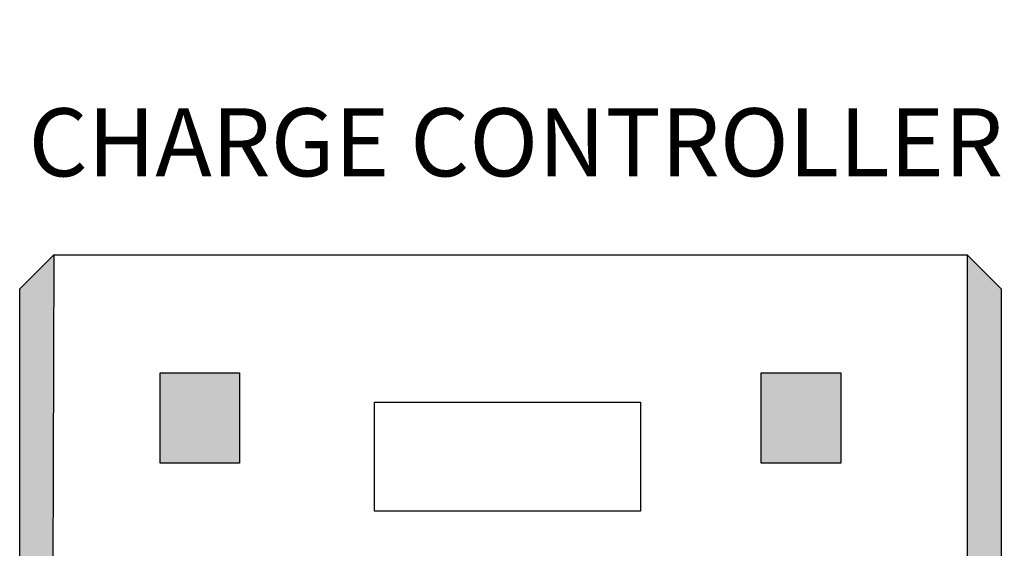
# Model space of a CAD drawing. Units: millimetres. Extents: x -8 to 285, y 5 to 221.
# Tile 7 of 30: x 26 to 84, y 82 to 113. Entities that reach past the tile are written whole.
import ezdxf

# ---------------------------------------------------------------- set-up
doc = ezdxf.new("R2010")
doc.units = ezdxf.units.MM
for name, color, linetype, lineweight in [('A-ANNO-DIMS', 2, 'Continuous', 18), ('E-ANNO-TEXT', 7, 'Continuous', 18), ('E-EQPM-PATT', 252, 'Continuous', 13), ('E-POWR-CTRL', 7, 'Continuous', 30)]:
    doc.layers.add(name, color=color, linetype=linetype, lineweight=lineweight)
doc.styles.get("Standard").update_dxf_attribs({"font": 'arial.ttf'})
doc.dimstyles.get("Standard").update_dxf_attribs({"dimtxt": 0.18, "dimasz": 0.18, "dimexe": 0.18, "dimexo": 0.0625, "dimgap": 0.09, "dimtad": 0, "dimtih": 1, "dimtoh": 1, "dimdec": 4, "dimzin": 0, "dimdsep": 46, "dimtxsty": 'Standard', "dimcen": 0.09, "dimadec": 0, "dimazin": 0, "dimtfac": 1, "dimtdec": 4, "dimtofl": 0, "dimtmove": 0, "dimatfit": 3, "dimfxl": 1, "dimtolj": 1, "dimtzin": 0, "dimarcsym": 0})

# ---------------------------------------------------------------- blocks, each defined once
blk = doc.blocks.new('*D10')
at = {"layer": 'A-ANNO-DIMS', "color": 0, "lineweight": -2, "transparency": 16777216}
for p, q in [((145.103, 206.457), (-7.608, 206.457)), ((-7.428, 206.277), (-7.428, 113.161)), ((-7.428, 19.682), (-7.428, 112.797)), ((30.453, 19.502), (-7.608, 19.502))]:
    blk.add_line(p, q, dxfattribs=at)
at = {"layer": 'A-ANNO-DIMS', "color": 0, "transparency": 16777216}
for points in [[(-7.458, 206.277), (-7.398, 206.277), (-7.428, 206.457)], [(-7.458, 19.682), (-7.398, 19.682), (-7.428, 19.502)]]:
    blk.add_solid(points, dxfattribs=at)
at = {"layer": 'Defpoints', "color": 0, "transparency": 16777216}
for p in [(-7.428, 206.457), (145.165, 206.457), (30.516, 19.502)]:
    blk.add_point(p, dxfattribs=at)
at = {"layer": 'A-ANNO-DIMS', "color": 0, "transparency": 16777216, "insert": (-7.428, 112.979), "char_height": 0.18, "attachment_point": 5}
blk.add_mtext('\\A1;186.95', dxfattribs=at)

msp = doc.modelspace()

# ---------------------------------------------------------------- hatches: boundary and pattern name
at = {"layer": 'E-EQPM-PATT'}
h = msp.add_hatch(color=256, dxfattribs=at)
h.set_gradient(color1=(248, 153, 30), color2=(248, 153, 30), tint=1)
h.paths.add_polyline_path([(28.1554, 99.1437), (26.1554, 97.1437), (26.1554, 65.7282), (28.0483, 63.8353)])
h.paths.add_polyline_path([(81.859, 63.7282), (83.859, 65.7282), (83.859, 97.1437), (81.859, 99.1437)])
h.paths.add_polyline_path([(39.086, 92.2191), (34.4177, 92.2191), (34.4177, 86.904), (39.086, 86.904)])
h.paths.add_polyline_path([(74.424, 86.904), (74.424, 92.2191), (69.7557, 92.2191), (69.7557, 86.904)])
h.paths.add_polyline_path([(74.5326, 81.2093), (69.8643, 81.2093), (69.8643, 75.8943), (74.5326, 75.8943)])
h.paths.add_polyline_path([(34.4177, 75.3519), (39.086, 75.3519), (39.086, 80.667), (34.4177, 80.667)])

# ---------------------------------------------------------------- linework, layer by layer
at = {"layer": 'E-POWR-CTRL'}
for p, q in [((28.1554, 99.1437), (28.0483, 63.8353)), ((81.859, 99.1437), (81.859, 63.7282))]:
    msp.add_line(p, q, dxfattribs=at)
for points in [[(28.1554, 99.1437), (81.859, 99.1437), (83.859, 97.1437), (83.859, 65.7282), (81.859, 63.7282), (28.1554, 63.7282), (26.1554, 65.7282), (26.1554, 97.1437)], [(34.4177, 92.2191), (39.086, 92.2191), (39.086, 86.904), (34.4177, 86.904)], [(69.7557, 92.2191), (74.424, 92.2191), (74.424, 86.904), (69.7557, 86.904)], [(47.0112, 90.4835), (62.6447, 90.4835), (62.6447, 84.0838), (47.0112, 84.0838)]]:
    msp.add_lwpolyline(points, close=True, dxfattribs=at)

# ---------------------------------------------------------------- texts
at = {"layer": 'E-ANNO-TEXT', "insert": (26.6766, 107.7676), "char_height": 4, "attachment_point": 1}
msp.add_mtext_dynamic_manual_height_columns('CHARGE CONTROLLER', width=66.795138, gutter_width=12.5, heights=[0], dxfattribs=at)

# ---------------------------------------------------------------- dimensions: what is measured, and where the dimension line sits
at = {"layer": 'A-ANNO-DIMS'}
dim = msp.add_linear_dim(base=(-7.4275, 206.4568), p1=(30.516, 19.502), p2=(145.1651, 206.4568), angle=90, dimstyle='Standard', override={"dimdec": 2, "dimlfac": 1, "dimrnd": 0, "dimzin": 0, "dimdsep": 46, "dimlunit": 2}, dxfattribs=at)
dim.commit()
dim.dimension.update_dxf_attribs({"geometry": '*D10', "text_midpoint": (-7.4275, 112.9794)})

doc.saveas('drawing.dxf')
